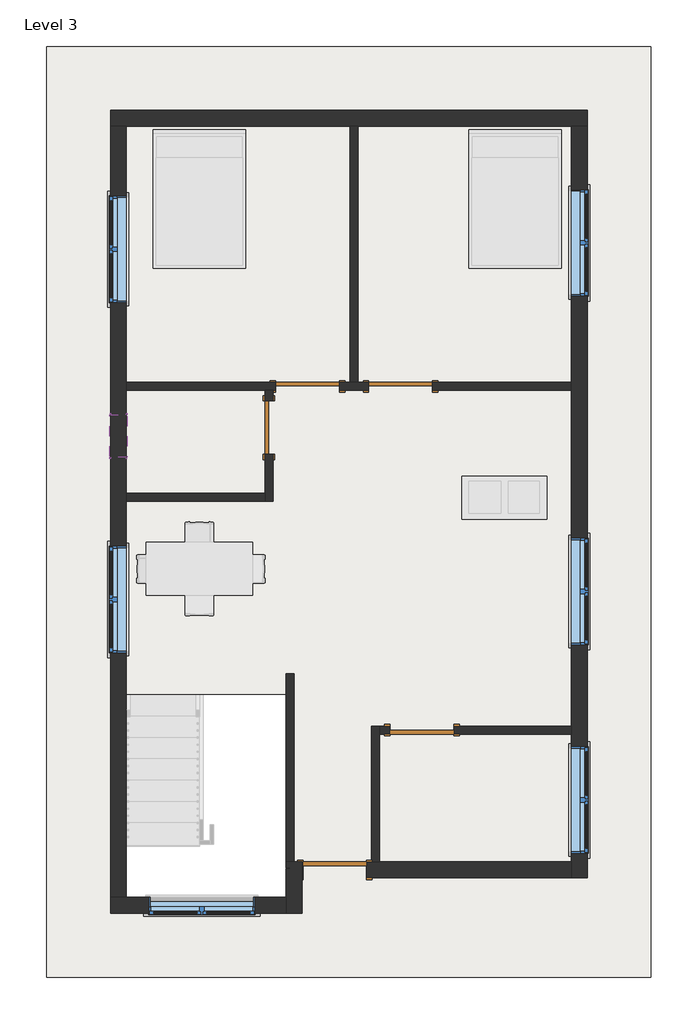
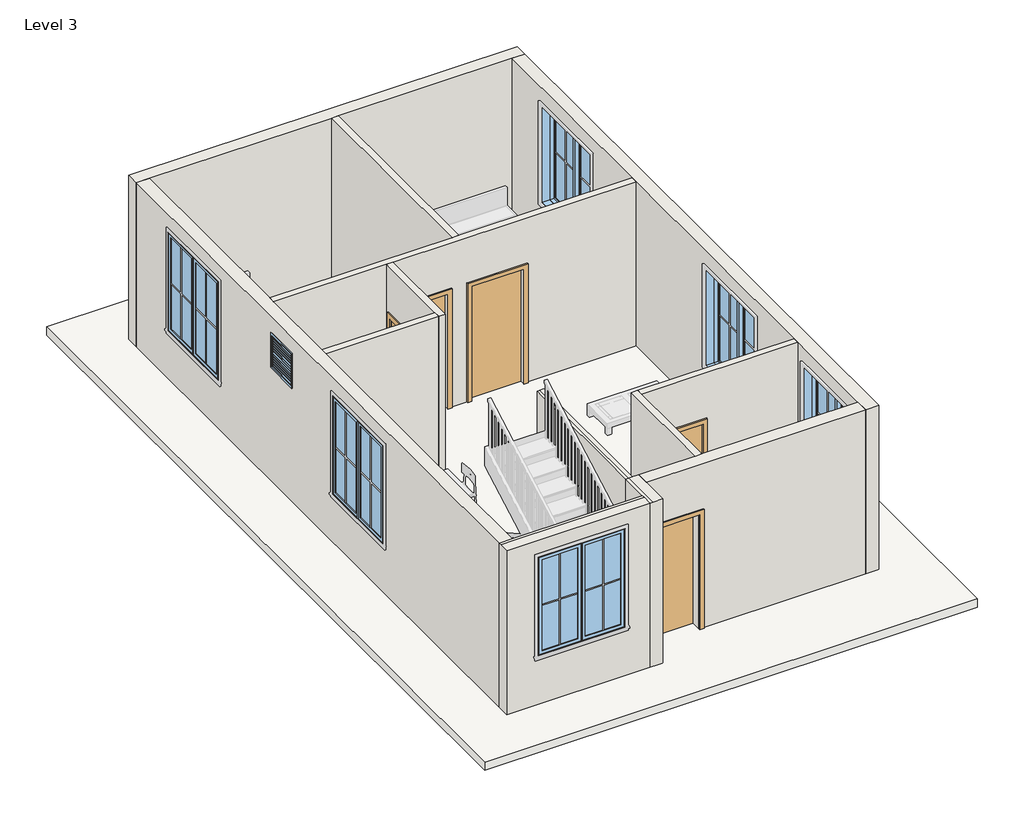
# One storey, part 1 of 3: 13 walls, 7 windows, 5 doors, 1 roof.
"""IFC4 building model written with IfcOpenShell, lengths in millimetres."""

from ifc_helpers import new_model, si_unit, frame, origin, place, context, project, spatial, polyline, outline, extrude, faceted_brep, transform, mapped, element, save
from components import door_214872d5, single_flush_door_3_e5f9f3c4, single_flush_door_3_305aa2a5, single_flush_door_3_0ca8825f, window_casement_double_win_5_f93960c7, window_f2d8fef0

model = new_model("IFC4")

# Units and contexts
model_context = context("Model", 3, world=origin())
ifc_project = project(units=[si_unit("LENGTHUNIT", "METRE", prefix="MILLI")], contexts=[model_context])

# Site, building, storey
site = spatial("IfcSite", under=ifc_project)
building = spatial("IfcBuilding", under=site)
storey = spatial("IfcBuildingStorey", under=building, Name="Level 3", Elevation=6248.4)

# Doors
placement = place(None, origin())
door_shape = door_214872d5(model_context)
element("IfcDoor", 1, ObjectType="Single-Flush : DOOR 2'6\"", at=placement, inside=storey, context=model_context, shape_type="MappedRepresentation", body=[
    mapped(door_shape, transform((-2193.930864, 251.0919982, 6248.4), x_axis=(0.0, 1.0, 0.0), y_axis=(-1.0, 0.0, 0.0), z_axis=(0.0, 0.0, 1.0))),
])
single_flush_door_3_shape = single_flush_door_3_e5f9f3c4(model_context)
element("IfcDoor", 2, ObjectType="Single-Flush : DOOR 3'", at=placement, inside=storey, context=model_context, shape_type="MappedRepresentation", body=[
    mapped(single_flush_door_3_shape, transform((-1641.3962678, 841.6419982, 6248.4), x_axis=(1.0, 0.0, 0.0), y_axis=(0.0, 1.0, 0.0), z_axis=(0.0, 0.0, 1.0))),
])
element("IfcDoor", 3, ObjectType="Single-Flush : DOOR 3'", at=placement, inside=storey, context=model_context, shape_type="MappedRepresentation", body=[
    mapped(single_flush_door_3_shape, transform((-3.180864, -4073.2580018, 6248.4), x_axis=(-1.0, 0.0, 0.0), y_axis=(0.0, -1.0, 0.0), z_axis=(0.0, 0.0, 1.0))),
])
single_flush_door_3_2_shape = single_flush_door_3_305aa2a5(model_context)
element("IfcDoor", 4, ObjectType="Single-Flush : DOOR 3'", at=placement, inside=storey, context=model_context, shape_type="MappedRepresentation", body=[
    mapped(single_flush_door_3_2_shape, transform((-307.980864, 841.6419982, 6248.4), x_axis=(-1.0, 0.0, 0.0), y_axis=(0.0, -1.0, 0.0), z_axis=(0.0, 0.0, 1.0))),
])
single_flush_door_3_3_shape = single_flush_door_3_0ca8825f(model_context)
element("IfcDoor", 5, ObjectType="Single-Flush : DOOR 3'", at=placement, inside=storey, context=model_context, shape_type="MappedRepresentation", body=[
    mapped(single_flush_door_3_3_shape, transform((-1250.955864, -6073.5080018, 6248.4), x_axis=(1.0, 0.0, 0.0), y_axis=(0.0, 1.0, 0.0), z_axis=(0.0, 0.0, 1.0))),
])

# Roof
element("IfcRoof", 6, ObjectType="ROOF 6\"", at=placement, inside=storey, context=model_context, shape_type="SweptSolid", body=[
    extrude(outline(polyline([(3273.419136, 5699.3919982), (3273.419136, -7610.2080018), (-5375.280864, -7610.2080018), (-5375.280864, 5699.3919982), (3273.419136, 5699.3919982)]), holes=[polyline([(-1895.480864, -3571.6080018), (-4232.280864, -3571.6080018), (-4232.280864, -6518.0080018), (-1895.480864, -6518.0080018), (-1895.480864, -3571.6080018)])]), frame((0.0, 0.0, 6096.0), z_axis=(0.0, 0.0, 1.0), x_axis=(1.0, 0.0, 0.0)), (0.0, 0.0, 1.0), 152.4),
])

# Walls
element("IfcWall", 7, ObjectType="WALL 4.5\"", at=placement, inside=storey, context=model_context, shape_type="SweptSolid", body=[
    extrude(outline(polyline([(-1031.880864, 898.7919982), (-1031.880864, 4556.3919982), (-917.580864, 4556.3919982), (-917.580864, 898.7919982), (-1031.880864, 898.7919982)])), frame((0.0, 0.0, 6248.4), z_axis=(0.0, 0.0, 1.0), x_axis=(1.0, 0.0, 0.0)), (0.0, 0.0, 1.0), 3048.0),
])
element("IfcWall", 8, ObjectType="WALL 4.5\"", at=placement, inside=storey, context=model_context, shape_type="Brep", body=[
    faceted_brep([(-765.180864, 898.7919982, 8382.0), (-765.180864, 898.7919982, 6248.4), (-917.580864, 898.7919982, 6248.4), (-1031.880864, 898.7919982, 6248.4), (-1184.1962678, 898.7919982, 6248.4), (-1184.1962678, 898.7919982, 8382.0), (-2098.5962678, 898.7919982, 8382.0), (-2098.5962678, 898.7919982, 6248.4), (-4232.280864, 898.7919982, 6248.4), (-4232.280864, 898.7919982, 9296.4), (-1031.880864, 898.7919982, 9296.4), (-917.580864, 898.7919982, 9296.4), (2130.419136, 898.7919982, 9296.4), (2130.419136, 898.7919982, 6248.4), (149.219136, 898.7919982, 6248.4), (149.219136, 898.7919982, 8382.0), (-1184.1962678, 784.4919982, 6248.4), (-765.180864, 784.4919982, 6248.4), (-765.180864, 784.4919982, 8382.0), (149.219136, 784.4919982, 8382.0), (149.219136, 784.4919982, 6248.4), (2130.419136, 784.4919982, 6248.4), (2130.419136, 784.4919982, 9296.4), (-2136.780864, 784.4919982, 9296.4), (-2251.080864, 784.4919982, 9296.4), (-4232.280864, 784.4919982, 9296.4), (-4232.280864, 784.4919982, 6248.4), (-2251.080864, 784.4919982, 6248.4), (-2136.780864, 784.4919982, 6248.4), (-2098.5962678, 784.4919982, 6248.4), (-2098.5962678, 784.4919982, 8382.0), (-1184.1962678, 784.4919982, 8382.0)], [[[0, 1, 2, 3, 4, 5, 6, 7, 8, 9, 10, 11, 12, 13, 14, 15]], [[16, 17, 18, 19, 20, 21, 22, 23, 24, 25, 26, 27, 28, 29, 30, 31]], [[29, 28, 27, 26, 8, 7]], [[14, 13, 21, 20]], [[4, 3, 2, 1, 17, 16]], [[13, 12, 22, 21]], [[9, 8, 26, 25]], [[5, 4, 16, 31]], [[6, 5, 31, 30]], [[7, 6, 30, 29]], [[18, 17, 1, 0]], [[19, 18, 0, 15]], [[20, 19, 15, 14]], [[12, 11, 10, 9, 25, 24, 23, 22]]]),
])
element("IfcWall", 9, ObjectType="WALL 4.5\"", at=placement, inside=storey, context=model_context, shape_type="Brep", body=[
    faceted_brep([(-2251.080864, 784.4919982, 6248.4), (-2251.080864, 632.0919982, 6248.4), (-2251.080864, 632.0919982, 8382.0), (-2251.080864, -129.9080018, 8382.0), (-2251.080864, -129.9080018, 6248.4), (-2251.080864, -688.7080018, 6248.4), (-2251.080864, -803.0080018, 6248.4), (-2251.080864, -803.0080018, 9296.4), (-2251.080864, -688.7080018, 9296.4), (-2251.080864, 784.4919982, 9296.4), (-2136.780864, 632.0919982, 8382.0), (-2136.780864, 632.0919982, 6248.4), (-2136.780864, 784.4919982, 6248.4), (-2136.780864, 784.4919982, 9296.4), (-2136.780864, -803.0080018, 9296.4), (-2136.780864, -803.0080018, 6248.4), (-2136.780864, -129.9080018, 6248.4), (-2136.780864, -129.9080018, 8382.0)], [[[0, 1, 2, 3, 4, 5, 6, 7, 8, 9]], [[10, 11, 12, 13, 14, 15, 16, 17]], [[16, 15, 6, 5, 4]], [[12, 11, 1, 0]], [[0, 9, 13, 12]], [[7, 6, 15, 14]], [[2, 1, 11, 10]], [[3, 2, 10, 17]], [[4, 3, 17, 16]], [[9, 8, 7, 14, 13]]]),
])
element("IfcWall", 10, ObjectType="WALL 4.5\"", at=placement, inside=storey, context=model_context, shape_type="SweptSolid", body=[
    extrude(outline(polyline([(-4232.280864, -688.7080018), (-2251.080864, -688.7080018), (-2251.080864, -803.0080018), (-4232.280864, -803.0080018), (-4232.280864, -688.7080018)])), frame((0.0, 0.0, 6248.4), z_axis=(0.0, 0.0, 1.0), x_axis=(1.0, 0.0, 0.0)), (0.0, 0.0, 1.0), 3048.0),
])
element("IfcWall", 11, ObjectType="WALL 4.5\"", at=placement, inside=storey, context=model_context, shape_type="Brep", body=[
    faceted_brep([(-1831.980864, -5959.2080018, 6248.4), (-1831.980864, -3266.8080018, 6248.4), (-1831.980864, -3266.8080018, 9296.4), (-1831.980864, -5959.2080018, 9296.4), (-1946.280864, -5959.2080018, 6248.4), (-1946.280864, -5959.2080018, 9296.4), (-1946.280864, -3266.8080018, 9296.4), (-1946.280864, -3266.8080018, 6248.4), (-1895.480864, -3266.8080018, 9296.4), (-1895.480864, -5959.2080018, 9296.4), (-1895.480864, -3571.6080018, 9296.4)], [[[0, 1, 2, 3]], [[4, 5, 6, 7]], [[1, 0, 4, 7]], [[2, 1, 7, 6, 8]], [[0, 3, 9, 5, 4]], [[3, 2, 8, 10, 9]], [[8, 6, 5, 9, 10]]]),
])
element("IfcWall", 12, ObjectType="WALL 4.5\"", at=placement, inside=storey, context=model_context, shape_type="Brep", body=[
    faceted_brep([(-612.780864, -5959.2080018, 6248.4), (-612.780864, -4130.4080018, 6248.4), (-612.780864, -4016.1080018, 6248.4), (-612.780864, -4016.1080018, 9296.4), (-612.780864, -4130.4080018, 9296.4), (-612.780864, -5959.2080018, 9296.4), (-727.080864, -5959.2080018, 6248.4), (-727.080864, -5959.2080018, 9296.4), (-727.080864, -4016.1080018, 9296.4), (-727.080864, -4016.1080018, 6248.4)], [[[0, 1, 2, 3, 4, 5]], [[6, 7, 8, 9]], [[2, 1, 0, 6, 9]], [[0, 5, 7, 6]], [[3, 2, 9, 8]], [[5, 4, 3, 8, 7]]]),
])
element("IfcWall", 13, ObjectType="WALL 4.5\"", at=placement, inside=storey, context=model_context, shape_type="SweptSolid", body=[
    extrude(outline(polyline([(6248.4, -612.780864), (6248.4, -460.380864), (8382.0, -460.380864), (8382.0, 454.019136), (6248.4, 454.019136), (6248.4, 2130.419136), (9296.4, 2130.419136), (9296.4, -612.780864), (6248.4, -612.780864)])), frame((0.0, -4130.4080018, 0.0), z_axis=(0.0, 1.0, 0.0), x_axis=(0.0, 0.0, 1.0)), (0.0, 0.0, 1.0), 114.3),
])
element("IfcWall", 14, ObjectType="WALL 9\"", at=placement, inside=storey, context=model_context, shape_type="Brep", body=[
    faceted_brep([(-4460.880864, 4556.3919982, 6248.4), (-4232.280864, 4556.3919982, 6248.4), (-1031.880864, 4556.3919982, 6248.4), (-917.580864, 4556.3919982, 6248.4), (2130.419136, 4556.3919982, 6248.4), (2359.019136, 4556.3919982, 6248.4), (2359.019136, 4556.3919982, 9296.4), (2130.419136, 4556.3919982, 9296.4), (-917.580864, 4556.3919982, 9296.4), (-1031.880864, 4556.3919982, 9296.4), (-4232.280864, 4556.3919982, 9296.4), (-4460.880864, 4556.3919982, 9296.4), (-4460.880864, 4784.9919982, 6248.4), (-4460.880864, 4784.9919982, 9296.4), (2359.019136, 4784.9919982, 9296.4), (2359.019136, 4784.9919982, 6248.4)], [[[0, 1, 2, 3, 4, 5, 6, 7, 8, 9, 10, 11]], [[12, 13, 14, 15]], [[5, 4, 3, 2, 1, 0, 12, 15]], [[6, 5, 15, 14]], [[0, 11, 13, 12]], [[11, 10, 9, 8, 7, 6, 14, 13]]]),
])
element("IfcWall", 15, ObjectType="WALL 9\"", at=placement, inside=storey, context=model_context, shape_type="Brep", body=[
    faceted_brep([(2130.419136, 4556.3919982, 6248.4), (2130.419136, 898.7919982, 6248.4), (2130.419136, 784.4919982, 6248.4), (2130.419136, -4016.1080018, 6248.4), (2130.419136, -4130.4080018, 6248.4), (2130.419136, -5959.2080018, 6248.4), (2130.419136, -6187.8080018, 6248.4), (2130.419136, -6187.8080018, 9296.4), (2130.419136, -5959.2080018, 9296.4), (2130.419136, -4130.4080018, 9296.4), (2130.419136, -4016.1080018, 9296.4), (2130.419136, 784.4919982, 9296.4), (2130.419136, 898.7919982, 9296.4), (2130.419136, 4556.3919982, 9296.4), (2130.419136, -5835.3830018, 8991.6), (2130.419136, -5835.3830018, 7162.8), (2130.419136, -4311.3830018, 7162.8), (2130.419136, -4311.3830018, 8991.6), (2130.419136, -2854.0580018, 8991.6), (2130.419136, -2854.0580018, 7162.8), (2130.419136, -1330.0580018, 7162.8), (2130.419136, -1330.0580018, 8991.6), (2130.419136, 2130.6919982, 8991.6), (2130.419136, 2130.6919982, 7162.8), (2130.419136, 3654.6919982, 7162.8), (2130.419136, 3654.6919982, 8991.6), (2359.019136, 4556.3919982, 6248.4), (2359.019136, 4556.3919982, 9296.4), (2359.019136, -6187.8080018, 9296.4), (2359.019136, -6187.8080018, 6248.4), (2359.019136, -5835.3830018, 8991.6), (2359.019136, -4311.3830018, 8991.6), (2359.019136, -4311.3830018, 7162.8), (2359.019136, -5835.3830018, 7162.8), (2359.019136, -2854.0580018, 8991.6), (2359.019136, -1330.0580018, 8991.6), (2359.019136, -1330.0580018, 7162.8), (2359.019136, -2854.0580018, 7162.8), (2359.019136, 2130.6919982, 8991.6), (2359.019136, 3654.6919982, 8991.6), (2359.019136, 3654.6919982, 7162.8), (2359.019136, 2130.6919982, 7162.8)], [[[0, 1, 2, 3, 4, 5, 6, 7, 8, 9, 10, 11, 12, 13], [14, 15, 16, 17], [18, 19, 20, 21], [22, 23, 24, 25]], [[26, 27, 28, 29], [30, 31, 32, 33], [34, 35, 36, 37], [38, 39, 40, 41]], [[6, 5, 4, 3, 2, 1, 0, 26, 29]], [[0, 13, 27, 26]], [[7, 6, 29, 28]], [[15, 14, 30, 33]], [[16, 15, 33, 32]], [[17, 16, 32, 31]], [[14, 17, 31, 30]], [[19, 18, 34, 37]], [[20, 19, 37, 36]], [[21, 20, 36, 35]], [[18, 21, 35, 34]], [[23, 22, 38, 41]], [[24, 23, 41, 40]], [[25, 24, 40, 39]], [[22, 25, 39, 38]], [[13, 12, 11, 10, 9, 8, 7, 28, 27]]]),
])
element("IfcWall", 16, ObjectType="WALL 9\"", at=placement, inside=storey, context=model_context, shape_type="Brep", body=[
    faceted_brep([(2130.419136, -5959.2080018, 6248.4), (-612.780864, -5959.2080018, 6248.4), (-727.080864, -5959.2080018, 6248.4), (-793.755864, -5959.2080018, 6248.4), (-793.755864, -5959.2080018, 8382.0), (-1708.155864, -5959.2080018, 8382.0), (-1708.155864, -5959.2080018, 6248.4), (-1717.680864, -5959.2080018, 6248.4), (-1717.680864, -5959.2080018, 9296.4), (-727.080864, -5959.2080018, 9296.4), (-612.780864, -5959.2080018, 9296.4), (2130.419136, -5959.2080018, 9296.4), (-793.755864, -6187.8080018, 8382.0), (-793.755864, -6187.8080018, 6248.4), (2130.419136, -6187.8080018, 6248.4), (2130.419136, -6187.8080018, 9296.4), (-1717.680864, -6187.8080018, 9296.4), (-1717.680864, -6187.8080018, 6248.4), (-1708.155864, -6187.8080018, 6248.4), (-1708.155864, -6187.8080018, 8382.0)], [[[0, 1, 2, 3, 4, 5, 6, 7, 8, 9, 10, 11]], [[12, 13, 14, 15, 16, 17, 18, 19]], [[18, 17, 7, 6]], [[14, 13, 3, 2, 1, 0]], [[0, 11, 15, 14]], [[8, 7, 17, 16]], [[4, 3, 13, 12]], [[5, 4, 12, 19]], [[6, 5, 19, 18]], [[11, 10, 9, 8, 16, 15]]]),
])
element("IfcWall", 17, ObjectType="WALL 9\"", at=placement, inside=storey, context=model_context, shape_type="Brep", body=[
    faceted_brep([(-1946.280864, -5959.2080018, 6248.4), (-1946.280864, -6467.2080018, 6248.4), (-1946.280864, -6695.8080018, 6248.4), (-1946.280864, -6695.8080018, 9296.4), (-1946.280864, -6467.2080018, 9296.4), (-1946.280864, -5959.2080018, 9296.4), (-1717.680864, -5959.2080018, 6248.4), (-1717.680864, -5959.2080018, 9296.4), (-1717.680864, -6187.8080018, 9296.4), (-1717.680864, -6695.8080018, 9296.4), (-1717.680864, -6695.8080018, 6248.4), (-1717.680864, -6187.8080018, 6248.4), (-1831.980864, -5959.2080018, 6248.4), (-1895.480864, -5959.2080018, 9296.4), (-1831.980864, -5959.2080018, 9296.4), (-1895.480864, -6695.8080018, 9296.4), (-1895.480864, -6518.0080018, 9296.4)], [[[0, 1, 2, 3, 4, 5]], [[6, 7, 8, 9, 10, 11]], [[2, 1, 0, 12, 6, 11, 10]], [[0, 5, 13, 14, 7, 6, 12]], [[3, 2, 10, 9, 15]], [[5, 4, 3, 15, 16, 13]], [[15, 9, 8, 7, 14, 13, 16]]]),
])
element("IfcWall", 18, ObjectType="WALL 9\"", at=placement, inside=storey, context=model_context, shape_type="Brep", body=[
    faceted_brep([(-1946.280864, -6467.2080018, 6248.4), (-4232.280864, -6467.2080018, 6248.4), (-4460.880864, -6467.2080018, 6248.4), (-4460.880864, -6467.2080018, 9296.4), (-4232.280864, -6467.2080018, 9296.4), (-1946.280864, -6467.2080018, 9296.4), (-3914.780864, -6467.2080018, 8991.6), (-3914.780864, -6467.2080018, 7162.8), (-2390.780864, -6467.2080018, 7162.8), (-2390.780864, -6467.2080018, 8991.6), (-1946.280864, -6695.8080018, 6248.4), (-1946.280864, -6695.8080018, 9296.4), (-4460.880864, -6695.8080018, 9296.4), (-4460.880864, -6695.8080018, 6248.4), (-3914.780864, -6695.8080018, 8991.6), (-2390.780864, -6695.8080018, 8991.6), (-2390.780864, -6695.8080018, 7162.8), (-3914.780864, -6695.8080018, 7162.8), (-1946.280864, -6518.0080018, 9296.4), (-4460.880864, -6518.0080018, 9296.4), (-4232.280864, -6518.0080018, 9296.4)], [[[0, 1, 2, 3, 4, 5], [6, 7, 8, 9]], [[10, 11, 12, 13], [14, 15, 16, 17]], [[2, 1, 0, 10, 13]], [[0, 5, 18, 11, 10]], [[3, 2, 13, 12, 19]], [[7, 6, 14, 17]], [[8, 7, 17, 16]], [[9, 8, 16, 15]], [[6, 9, 15, 14]], [[5, 4, 3, 19, 20, 18]], [[19, 12, 11, 18, 20]]]),
])
element("IfcWall", 19, ObjectType="WALL 9\"", at=placement, inside=storey, context=model_context, shape_type="Brep", body=[
    faceted_brep([(-4232.280864, -6467.2080018, 6248.4), (-4232.280864, -803.0080018, 6248.4), (-4232.280864, -688.7080018, 6248.4), (-4232.280864, 784.4919982, 6248.4), (-4232.280864, 898.7919982, 6248.4), (-4232.280864, 4556.3919982, 6248.4), (-4232.280864, 4556.3919982, 9296.4), (-4232.280864, 898.7919982, 9296.4), (-4232.280864, 784.4919982, 9296.4), (-4232.280864, -688.7080018, 9296.4), (-4232.280864, -803.0080018, 9296.4), (-4232.280864, -3571.6080018, 9296.4), (-4232.280864, -6467.2080018, 9296.4), (-4232.280864, -1445.1400081, 8991.6), (-4232.280864, -1445.1400081, 7162.8), (-4232.280864, -2969.1400081, 7162.8), (-4232.280864, -2969.1400081, 8991.6), (-4232.280864, 3562.6287133, 8991.6), (-4232.280864, 3562.6287133, 7162.8), (-4232.280864, 2038.6287133, 7162.8), (-4232.280864, 2038.6287133, 8991.6), (-4232.280864, -174.3580018, 8991.6), (-4232.280864, 435.2419982, 8991.6), (-4232.280864, 435.2419982, 8382.0), (-4232.280864, -174.3580018, 8382.0), (-4460.880864, -6467.2080018, 6248.4), (-4460.880864, -6467.2080018, 9296.4), (-4460.880864, 4556.3919982, 9296.4), (-4460.880864, 4556.3919982, 6248.4), (-4460.880864, -1445.1400081, 8991.6), (-4460.880864, -2969.1400081, 8991.6), (-4460.880864, -2969.1400081, 7162.8), (-4460.880864, -1445.1400081, 7162.8), (-4460.880864, 3562.6287133, 8991.6), (-4460.880864, 2038.6287133, 8991.6), (-4460.880864, 2038.6287133, 7162.8), (-4460.880864, 3562.6287133, 7162.8), (-4460.880864, -174.3580018, 8991.6), (-4460.880864, -174.3580018, 8382.0), (-4460.880864, 435.2419982, 8382.0), (-4460.880864, 435.2419982, 8991.6)], [[[0, 1, 2, 3, 4, 5, 6, 7, 8, 9, 10, 11, 12], [13, 14, 15, 16], [17, 18, 19, 20], [21, 22, 23, 24]], [[25, 26, 27, 28], [29, 30, 31, 32], [33, 34, 35, 36], [37, 38, 39, 40]], [[5, 4, 3, 2, 1, 0, 25, 28]], [[6, 5, 28, 27]], [[0, 12, 26, 25]], [[14, 13, 29, 32]], [[15, 14, 32, 31]], [[16, 15, 31, 30]], [[13, 16, 30, 29]], [[18, 17, 33, 36]], [[19, 18, 36, 35]], [[20, 19, 35, 34]], [[17, 20, 34, 33]], [[38, 37, 21, 24]], [[39, 38, 24, 23]], [[40, 39, 23, 22]], [[37, 40, 22, 21]], [[12, 11, 10, 9, 8, 7, 6, 27, 26]]]),
])

# Windows
window_casement_double_win_5_shape = window_casement_double_win_5_f93960c7(model_context)
element("IfcWindow", 20, ObjectType="Window-Casement-Double : WIN 5'", at=placement, inside=storey, context=model_context, shape_type="MappedRepresentation", body=[
    mapped(window_casement_double_win_5_shape, transform((-3152.780864, -6581.5080018, 6248.4), x_axis=(-1.0, 0.0, 0.0), y_axis=(0.0, -1.0, 0.0), z_axis=(0.0, 0.0, 1.0))),
])
element("IfcWindow", 21, ObjectType="Window-Casement-Double : WIN 5'", at=placement, inside=storey, context=model_context, shape_type="MappedRepresentation", body=[
    mapped(window_casement_double_win_5_shape, transform((2244.719136, -5073.3830018, 6248.4), x_axis=(0.0, -1.0, 0.0), y_axis=(1.0, 0.0, 0.0), z_axis=(0.0, 0.0, 1.0))),
])
element("IfcWindow", 22, ObjectType="Window-Casement-Double : WIN 5'", at=placement, inside=storey, context=model_context, shape_type="MappedRepresentation", body=[
    mapped(window_casement_double_win_5_shape, transform((2244.719136, -2092.0580018, 6248.4), x_axis=(0.0, -1.0, 0.0), y_axis=(1.0, 0.0, 0.0), z_axis=(0.0, 0.0, 1.0))),
])
element("IfcWindow", 23, ObjectType="Window-Casement-Double : WIN 5'", at=placement, inside=storey, context=model_context, shape_type="MappedRepresentation", body=[
    mapped(window_casement_double_win_5_shape, transform((-4346.580864, -2207.1400081, 6248.4), x_axis=(0.0, 1.0, 0.0), y_axis=(-1.0, 0.0, 0.0), z_axis=(0.0, 0.0, 1.0))),
])
element("IfcWindow", 24, ObjectType="Window-Casement-Double : WIN 5'", at=placement, inside=storey, context=model_context, shape_type="MappedRepresentation", body=[
    mapped(window_casement_double_win_5_shape, transform((2244.719136, 2892.6919982, 6248.4), x_axis=(0.0, -1.0, 0.0), y_axis=(1.0, 0.0, 0.0), z_axis=(0.0, 0.0, 1.0))),
])
element("IfcWindow", 25, ObjectType="Window-Casement-Double : WIN 5'", at=placement, inside=storey, context=model_context, shape_type="MappedRepresentation", body=[
    mapped(window_casement_double_win_5_shape, transform((-4346.580864, 2800.6287133, 6248.4), x_axis=(0.0, 1.0, 0.0), y_axis=(-1.0, 0.0, 0.0), z_axis=(0.0, 0.0, 1.0))),
])
window_shape = window_f2d8fef0(model_context)
element("IfcWindow", 26, ObjectType="Window-Louvers : 24\" x 24\"", at=placement, inside=storey, context=model_context, shape_type="MappedRepresentation", body=[
    mapped(window_shape, transform((-4352.930864, 130.4419982, 7467.6), x_axis=(0.0, 1.0, 0.0), y_axis=(-1.0, 0.0, 0.0), z_axis=(0.0, 0.0, 1.0))),
])

save(model, "model.ifc")

# Revit data of these elements
# Type "Single-Flush : DOOR 2'6\""
#   Type Mark = "9"
#   Construction Type Id = "MDOOR"
#   Assembly Code = "C1020"
#   Analytic Construction = "Metal"
#   Thickness = 0' - 2"
#   Heat Transfer Coefficient (U) = 0.651978 BTU/(h·ft²·°F)
#   Height = 7' - 0"
#   Trim Projection Ext = 0' - 1"
#   Trim Projection Int = 0' - 1"
#   Trim Width = 0' - 3"
#   Width = 2' - 6"
#   Define Thermal Properties by = 1
#   Door Material = Door - Panel
#   Frame Material = Door - Frame
#   Visual Light Transmittance = 0
#   Solar Heat Gain Coefficient = 0
#   Function = (empty or 0)
#   Wall Closure = (empty or 0)
# Type "Single-Flush : DOOR 3'"
#   Type Mark = "8"
#   Construction Type Id = "MDOOR"
#   Assembly Code = "C1020"
#   Analytic Construction = "Metal"
#   Thickness = 0' - 2"
#   Heat Transfer Coefficient (U) = 0.651978 BTU/(h·ft²·°F)
#   Height = 7' - 0"
#   Trim Projection Ext = 0' - 1"
#   Trim Projection Int = 0' - 1"
#   Trim Width = 0' - 3"
#   Width = 3' - 0"
#   Define Thermal Properties by = 1
#   Door Material = Door - Panel
#   Frame Material = Door - Frame
#   Visual Light Transmittance = 0
#   Solar Heat Gain Coefficient = 0
#   Function = (empty or 0)
#   Wall Closure = (empty or 0)
# Type "ROOF 6\""
#   Assembly Code = "B1020"
#   Layers, outside or top first: 0' - 6" no material (function 1)
# Type "WALL 4.5\""
#   Assembly Code = "B2010"
#   Layers, outside or top first: 0' - 4 1/2" no material (function 1)
# Type "WALL 9\""
#   Assembly Code = "B2010"
#   Layers, outside or top first: 0' - 9" no material (function 1)
# Type "Window-Casement-Double : WIN 5'"
#   Type Mark = "18"
#   Fire Rating = "0.5h"
#   Assembly Code = "B2020100"
#   Analytic Construction = "Double glazing - domestic"
#   Frame Extension [instance default] = 0' - 0 1/4"
#   Window Inset [instance default] = 0' - 0"
#   Wall Thickness [instance default] = 0' - 6"
#   Interior Wall Closure [instance default] = 0' - 2 1/4"
#   Half Width = 2' - 6"
#   Visual Light Transmittance = 0.81
#   Thermal Resistance (R) = 1.8146 (h·ft²·°F)/BTU
#   Solar Heat Gain Coefficient = 0.76
#   Rough Width = 5' - 0 1/2"
#   Rough Height = 6' - 0 1/2"
#   Height = 6' - 0"
#   Heat Transfer Coefficient (U) = 0.5511 BTU/(h·ft²·°F)
#   Exterior Wall Closure [instance default] = 0' - 1 1/4"
#   Extension Jamb [instance default] = 0' - 2 1/4"
#   Default Sill Height = 3' - 0"
#   Width = 5' - 0"
#   Muntin Visibility = yes
#   Interior Trim Visibility [instance default] = yes
#   Exterior Trim Visibility [instance default] = yes
#   Extension Jamb Visibility [instance default] = yes
#   Interior Trim Material = Wood - Stained
#   Muntin Pattern = Muntin Pattern_2x2 : Muntin Pattern_2x2
#   Interior Trim = Trim-Window-Interior-Flat : Picture Frame
#   Interior Frame Material = Wood - Stained
#   Glass Panel Material = Glass
#   Exterior Trim Material = Clad - White
#   Exterior Trim = Trim-Window-Exterior-Flat : with Sill
#   Exterior Frame Material = Clad - White
#   Wall Closure = (empty or 0)
# Type "Window-Louvers : 24\" x 24\""
#   Type Mark = "19"
#   Construction Type Id = "GSP4R"
#   Assembly Code = "B20"
#   Analytic Construction = "1/8 in Pilkington single glazing"
#   Visual Light Transmittance = 0.9
#   Thermal Resistance (R) = 1.53941 (h·ft²·°F)/BTU
#   Solar Heat Gain Coefficient = 0.78
#   Max Height = 1' - 11.74264"
#   Height = 2' - 0"
#   Heat Transfer Coefficient (U) = 0.6496 BTU/(h·ft²·°F)
#   Blade Width [instance default] = 1' - 10 1/2"
#   Blade Vertical Thickness = 0' - 0.35355"
#   Blade Thickness = 0' - 0 1/4"
#   Blade Spacing = 0' - 1 1/2"
#   Blade Height = 0' - 1.85355"
#   Blade Depth = 0' - 3"
#   Blade Angle = 45.00°
#   Default Sill Height = 3' - 0"
#   Trim Projection_Exterior = 0' - 0 1/2"
#   Trim Projection_Interior = 0' - 0 1/2"
#   Trim Width_Exterior = 0' - 1 1/2"
#   Trim Width_Interior = 0' - 1 1/2"
#   Width = 2' - 0"
#   Max Blade Count = 12
#   Define Thermal Properties by = 1
#   Blade Count = 12
#   Frame Material = Birch
#   Louver Material = Birch
#   Trim Exterior Material = Birch
#   Trim Interior Material = Birch
#   Wall Closure = (empty or 0)
# Element 1 (IfcDoor, "Single-Flush : DOOR 2'6\"")
#   Phase Created = New Construction
#   Materials on its faces: "Door - Frame", "Door - Panel"
# Elements 2, 3, 4, 5 (IfcDoor, "Single-Flush : DOOR 3'")
#   Phase Created = New Construction
#   Materials on its faces: "Door - Frame", "Door - Panel"
# Element 6 (IfcRoof, "ROOF 6\"")
#   built-in parameter 1001705 = 20.5 (stored number, unit not read)
#   built-in parameter 1001701 = -0.5 (stored number, unit not read)
#   built-in parameter 1001710 = 33615
#   Phase Created = New Construction
#   Materials on its faces: "Copper", "Wood - Stained"
# Elements 7, 8, 9, 10, 12, 13 (IfcWall, "WALL 4.5\"")
#   Top Offset = 0' - 0"
#   Base Offset = 0' - 0"
#   Unconnected Height = 10' - 0"
#   wall height = 10' - 0"
#   Phase Created = New Construction
#   Base Constraint = Level 3
#   Materials on its faces: "Default Wall"
# Element 11 (IfcWall, "WALL 4.5\"")
#   Top Offset = 0' - 0"
#   Base Offset = 0' - 0"
#   Unconnected Height = 10' - 0"
#   wall height = 10' - 0"
#   Phase Created = New Construction
#   Base Constraint = Level 3
#   Materials on its faces: "Default Wall", "Copper"
# Elements 14, 15, 16 (IfcWall, "WALL 9\"")
#   Top Offset = 0' - 0"
#   Base Offset = 0' - 0"
#   Unconnected Height = 10' - 0"
#   wall height = 10' - 0"
#   Phase Created = New Construction
#   Base Constraint = Level 3
#   Materials on its faces: "Default Wall"
# Elements 17, 18, 19 (IfcWall, "WALL 9\"")
#   Top Offset = 0' - 0"
#   Base Offset = 0' - 0"
#   Unconnected Height = 10' - 0"
#   wall height = 10' - 0"
#   Phase Created = New Construction
#   Base Constraint = Level 3
#   Materials on its faces: "Default Wall", "Copper"
# Element 20 (IfcWindow, "Window-Casement-Double : WIN 5'")
#   Mark = "15"
#   Window Inset = 0' - 0"
#   Interior Wall Closure = 0' - 2 1/4"
#   Frame Extension = 0' - 0 1/4"
#   Exterior Wall Closure = 0' - 1 1/4"
#   Interior Trim Visibility = yes
#   Exterior Trim Visibility = yes
#   Phase Created = New Construction
#   Materials on its faces: "Wood - Stained", "Glass", "Clad - White"
# Element 21 (IfcWindow, "Window-Casement-Double : WIN 5'")
#   Mark = "16"
#   Window Inset = 0' - 0"
#   Interior Wall Closure = 0' - 2 1/4"
#   Frame Extension = 0' - 0 1/4"
#   Exterior Wall Closure = 0' - 1 1/4"
#   Interior Trim Visibility = yes
#   Exterior Trim Visibility = yes
#   Phase Created = New Construction
#   Materials on its faces: "Wood - Stained", "Glass", "Clad - White"
# Element 22 (IfcWindow, "Window-Casement-Double : WIN 5'")
#   Mark = "17"
#   Window Inset = 0' - 0"
#   Interior Wall Closure = 0' - 2 1/4"
#   Frame Extension = 0' - 0 1/4"
#   Exterior Wall Closure = 0' - 1 1/4"
#   Interior Trim Visibility = yes
#   Exterior Trim Visibility = yes
#   Phase Created = New Construction
#   Materials on its faces: "Wood - Stained", "Glass", "Clad - White"
# Element 23 (IfcWindow, "Window-Casement-Double : WIN 5'")
#   Mark = "18"
#   Window Inset = 0' - 0"
#   Interior Wall Closure = 0' - 2 1/4"
#   Frame Extension = 0' - 0 1/4"
#   Exterior Wall Closure = 0' - 1 1/4"
#   Interior Trim Visibility = yes
#   Exterior Trim Visibility = yes
#   Phase Created = New Construction
#   Materials on its faces: "Wood - Stained", "Glass", "Clad - White"
# Element 24 (IfcWindow, "Window-Casement-Double : WIN 5'")
#   Mark = "19"
#   Window Inset = 0' - 0"
#   Interior Wall Closure = 0' - 2 1/4"
#   Frame Extension = 0' - 0 1/4"
#   Exterior Wall Closure = 0' - 1 1/4"
#   Interior Trim Visibility = yes
#   Exterior Trim Visibility = yes
#   Phase Created = New Construction
#   Materials on its faces: "Wood - Stained", "Glass", "Clad - White"
# Element 25 (IfcWindow, "Window-Casement-Double : WIN 5'")
#   Mark = "20"
#   Window Inset = 0' - 0"
#   Interior Wall Closure = 0' - 2 1/4"
#   Frame Extension = 0' - 0 1/4"
#   Exterior Wall Closure = 0' - 1 1/4"
#   Interior Trim Visibility = yes
#   Exterior Trim Visibility = yes
#   Phase Created = New Construction
#   Materials on its faces: "Wood - Stained", "Glass", "Clad - White"
# Element 26 (IfcWindow, "Window-Louvers : 24\" x 24\"")
#   Mark = "21"
#   Blade Width = 1' - 10 1/2"
#   Phase Created = New Construction
#   Materials on its faces: "Birch"
# Materials
#   "Door - Panel": class "Wood", colour RGB 210 159 95, transparency 0, Cost = 0
#   "Door - Frame": colour RGB 118 70 51, transparency 0, Cost = 0
#   "Wood - Stained": class "Wood", colour RGB 224 178 126, transparency 0, Cost = 0
#   "Glass": class "Glass", colour RGB 0 128 192, transparency 0.75, Description = "Soda Lime Glass", Cost = 0
#   "Clad - White": class "Wood", colour RGB 242 242 238, transparency 0, Cost = 0
#   "Birch": class "Wood", colour RGB 224 178 126, transparency 0, Description = "Betula Alleghaniensis", Cost = 0
#   "Copper": class "Metal", colour RGB 0 0 0, transparency 0, Description = "Copper, matte finish", Cost = 0
#   "Default Wall": colour RGB 128 128 128, transparency 0, Cost = 0
